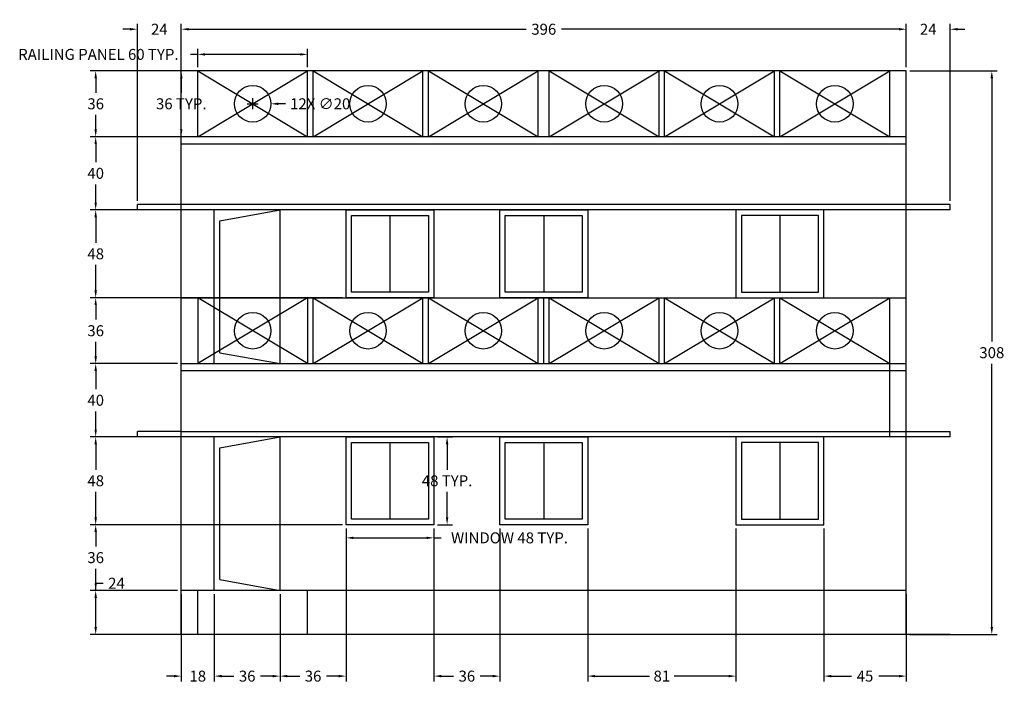
# Model space of a CAD drawing. Units: inches. Extents: x 853 to 2068, y 1026 to 2097.
# Tile 3 of 6: x 856 to 1394, y 1735 to 2097. Entities that reach past the tile are written whole.
import ezdxf

# ---------------------------------------------------------------- set-up
doc = ezdxf.new("R2010")
doc.units = ezdxf.units.IN
doc.header["$MEASUREMENT"] = 0
doc.layers.add('A-ANNO-DIMS', color=2, linetype='Continuous', lineweight=18)
doc.layers.add('A-ELEV', color=7, linetype='Continuous', lineweight=25)
doc.styles.get("Standard").update_dxf_attribs({"font": 'arial.ttf'})
doc.dimstyles.get("Standard").update_dxf_attribs({"dimtxt": 6, "dimasz": 4, "dimexe": 3, "dimexo": 2, "dimgap": 3, "dimtad": 0, "dimtih": 1, "dimtoh": 1, "dimdec": 0, "dimzin": 0, "dimdsep": 46, "dimlunit": 3, "dimtxsty": 'Standard', "dimcen": 3, "dimadec": 0, "dimazin": 0, "dimtfac": 1, "dimtdec": 0, "dimtofl": 0, "dimtmove": 0, "dimatfit": 3, "dimfxl": 1, "dimtolj": 1, "dimtzin": 0, "dimarcsym": 0})

# ---------------------------------------------------------------- blocks, each defined once
blk = doc.blocks.new('RAIL-PANEL')
for p, q in [((0, 36), (0, 0)), ((60, 36), (0, 0)), ((60, 0), (0, 36)), ((60, 36), (60, 0))]:
    blk.add_line(p, q)
blk.add_circle((30, 18), 10)
blk = doc.blocks.new('WIN-ELEV')
blk.add_line((24, 45), (24, 3))
for points in [[(0, 48), (48, 48), (48, 0), (0, 0)], [(3, 45), (45, 45), (45, 3), (3, 3)]]:
    blk.add_lwpolyline(points, close=True)
blk = doc.blocks.new('*D9')
at = {"layer": 'A-ANNO-DIMS', "color": 0, "lineweight": -2, "transparency": 16777216}
for p, q in [((1034.75, 1819.25), (1034.75, 1811.05)), ((1082.75, 1819.25), (1082.75, 1811.05)), ((1038.75, 1814.05), (1078.75, 1814.05)), ((1082.75, 1814.05), (1086.75, 1814.05))]:
    blk.add_line(p, q, dxfattribs=at)
at = {"layer": 'A-ANNO-DIMS', "color": 0, "transparency": 16777216}
for points in [[(1038.75, 1814.72), (1038.75, 1813.38), (1034.75, 1814.05)], [(1078.75, 1814.72), (1078.75, 1813.38), (1082.75, 1814.05)]]:
    blk.add_solid(points, dxfattribs=at)
at = {"layer": 'Defpoints', "color": 0, "transparency": 16777216}
for p in [(1034.75, 1821.25), (1082.75, 1821.25), (1082.75, 1814.05)]:
    blk.add_point(p, dxfattribs=at)
at = {"layer": 'A-ANNO-DIMS', "color": 0, "transparency": 16777216, "insert": (1124.03, 1814.05), "char_height": 6, "attachment_point": 5}
blk.add_mtext('\\A1;WINDOW 48 TYP.', dxfattribs=at)
blk = doc.blocks.new('*D10')
at = {"layer": 'A-ANNO-DIMS', "color": 0, "lineweight": -2, "transparency": 16777216}
for p, q in [((1084.75, 1869.25), (1092.95, 1869.25)), ((1089.95, 1865.25), (1089.95, 1851.31)), ((1089.95, 1825.25), (1089.95, 1839.19)), ((1084.75, 1821.25), (1092.95, 1821.25))]:
    blk.add_line(p, q, dxfattribs=at)
at = {"layer": 'A-ANNO-DIMS', "color": 0, "transparency": 16777216}
for points in [[(1089.28, 1865.25), (1090.62, 1865.25), (1089.95, 1869.25)], [(1089.28, 1825.25), (1090.62, 1825.25), (1089.95, 1821.25)]]:
    blk.add_solid(points, dxfattribs=at)
at = {"layer": 'Defpoints', "color": 0, "transparency": 16777216}
for p in [(1082.75, 1869.25), (1089.95, 1869.25), (1082.75, 1821.25)]:
    blk.add_point(p, dxfattribs=at)
at = {"layer": 'A-ANNO-DIMS', "color": 0, "transparency": 16777216, "insert": (1089.95, 1845.25), "char_height": 6, "attachment_point": 5}
blk.add_mtext('\\A1;48 TYP.', dxfattribs=at)
blk = doc.blocks.new('*D11')
at = {"layer": 'A-ANNO-DIMS', "color": 0, "lineweight": -2, "transparency": 16777216}
for p, q in [((953.75, 2078.25), (949.75, 2078.25)), ((953.75, 2071.25), (953.75, 2081.25)), ((1009.75, 2078.25), (957.75, 2078.25)), ((1013.75, 2071.25), (1013.75, 2081.25))]:
    blk.add_line(p, q, dxfattribs=at)
at = {"layer": 'A-ANNO-DIMS', "color": 0, "transparency": 16777216}
for points in [[(957.75, 2078.92), (957.75, 2077.58), (953.75, 2078.25)], [(1009.75, 2078.92), (1009.75, 2077.58), (1013.75, 2078.25)]]:
    blk.add_solid(points, dxfattribs=at)
at = {"layer": 'Defpoints', "color": 0, "transparency": 16777216}
for p in [(953.75, 2078.25), (953.75, 2069.25), (1013.75, 2069.25)]:
    blk.add_point(p, dxfattribs=at)
at = {"layer": 'A-ANNO-DIMS', "color": 0, "transparency": 16777216, "insert": (899.46, 2078.25), "char_height": 6, "attachment_point": 5}
blk.add_mtext('\\A1;RAILING PANEL 60 TYP.', dxfattribs=at)
blk = doc.blocks.new('*D12')
at = {"layer": 'A-ANNO-DIMS', "color": 0, "lineweight": -2, "transparency": 16777216}
for p, q in [((951.75, 2069.25), (941.75, 2069.25)), ((944.75, 2065.25), (944.75, 2057.32)), ((944.75, 2037.25), (944.75, 2045.19)), ((951.75, 2033.25), (941.75, 2033.25))]:
    blk.add_line(p, q, dxfattribs=at)
at = {"layer": 'A-ANNO-DIMS', "color": 0, "transparency": 16777216}
for points in [[(944.08, 2065.25), (945.42, 2065.25), (944.75, 2069.25)], [(944.08, 2037.25), (945.42, 2037.25), (944.75, 2033.25)]]:
    blk.add_solid(points, dxfattribs=at)
at = {"layer": 'Defpoints', "color": 0, "transparency": 16777216}
for p in [(953.75, 2069.25), (944.75, 2033.25), (953.75, 2033.25)]:
    blk.add_point(p, dxfattribs=at)
at = {"layer": 'A-ANNO-DIMS', "color": 0, "transparency": 16777216, "insert": (944.75, 2051.25), "char_height": 6, "attachment_point": 5}
blk.add_mtext('\\A1;36 TYP.', dxfattribs=at)
blk = doc.blocks.new('*D76')
at = {"layer": 'A-ANNO-DIMS', "color": 0, "lineweight": -2, "transparency": 16777216}
for p, q in [((898, 1785.25), (898, 1789.25)), ((898, 1789.25), (902, 1789.25)), ((942.75, 1785.25), (895, 1785.25)), ((898, 1765.25), (898, 1781.25)), ((942.75, 1761.25), (895, 1761.25))]:
    blk.add_line(p, q, dxfattribs=at)
at = {"layer": 'A-ANNO-DIMS', "color": 0, "transparency": 16777216}
for points in [[(897.33, 1781.25), (898.67, 1781.25), (898, 1785.25)], [(897.33, 1765.25), (898.67, 1765.25), (898, 1761.25)]]:
    blk.add_solid(points, dxfattribs=at)
at = {"layer": 'Defpoints', "color": 0, "transparency": 16777216}
for p in [(898, 1785.25), (944.75, 1785.25), (944.75, 1761.25)]:
    blk.add_point(p, dxfattribs=at)
at = {"layer": 'A-ANNO-DIMS', "color": 0, "transparency": 16777216, "insert": (909.34, 1789.25), "char_height": 6, "attachment_point": 5}
blk.add_mtext('\\A1;24', dxfattribs=at)
blk = doc.blocks.new('*D77')
at = {"layer": 'A-ANNO-DIMS', "color": 0, "lineweight": -2, "transparency": 16777216}
for p, q in [((1032.75, 1821.25), (895, 1821.25)), ((898, 1817.25), (898, 1809.32)), ((898, 1789.25), (898, 1797.19)), ((942.75, 1785.25), (895, 1785.25))]:
    blk.add_line(p, q, dxfattribs=at)
at = {"layer": 'A-ANNO-DIMS', "color": 0, "transparency": 16777216}
for points in [[(897.33, 1817.25), (898.67, 1817.25), (898, 1821.25)], [(897.33, 1789.25), (898.67, 1789.25), (898, 1785.25)]]:
    blk.add_solid(points, dxfattribs=at)
at = {"layer": 'Defpoints', "color": 0, "transparency": 16777216}
for p in [(898, 1821.25), (1034.75, 1821.25), (944.75, 1785.25)]:
    blk.add_point(p, dxfattribs=at)
at = {"layer": 'A-ANNO-DIMS', "color": 0, "transparency": 16777216, "insert": (898, 1803.25), "char_height": 6, "attachment_point": 5}
blk.add_mtext('\\A1;36', dxfattribs=at)
blk = doc.blocks.new('*D78')
at = {"layer": 'A-ANNO-DIMS', "color": 0, "lineweight": -2, "transparency": 16777216}
for p, q in [((942.75, 1869.25), (895, 1869.25)), ((898, 1865.25), (898, 1851.31)), ((898, 1825.25), (898, 1839.19)), ((1032.75, 1821.25), (895, 1821.25))]:
    blk.add_line(p, q, dxfattribs=at)
at = {"layer": 'A-ANNO-DIMS', "color": 0, "transparency": 16777216}
for points in [[(897.33, 1865.25), (898.67, 1865.25), (898, 1869.25)], [(897.33, 1825.25), (898.67, 1825.25), (898, 1821.25)]]:
    blk.add_solid(points, dxfattribs=at)
at = {"layer": 'Defpoints', "color": 0, "transparency": 16777216}
for p in [(898, 1869.25), (944.75, 1869.25), (1034.75, 1821.25)]:
    blk.add_point(p, dxfattribs=at)
at = {"layer": 'A-ANNO-DIMS', "color": 0, "transparency": 16777216, "insert": (898, 1845.25), "char_height": 6, "attachment_point": 5}
blk.add_mtext('\\A1;48', dxfattribs=at)
blk = doc.blocks.new('*D79')
at = {"layer": 'A-ANNO-DIMS', "color": 0, "lineweight": -2, "transparency": 16777216}
for p, q in [((942.75, 1909.25), (895, 1909.25)), ((898, 1905.25), (898, 1895.31)), ((898, 1873.25), (898, 1883.19)), ((942.75, 1869.25), (895, 1869.25))]:
    blk.add_line(p, q, dxfattribs=at)
at = {"layer": 'A-ANNO-DIMS', "color": 0, "transparency": 16777216}
for points in [[(897.33, 1905.25), (898.67, 1905.25), (898, 1909.25)], [(897.33, 1873.25), (898.67, 1873.25), (898, 1869.25)]]:
    blk.add_solid(points, dxfattribs=at)
at = {"layer": 'Defpoints', "color": 0, "transparency": 16777216}
for p in [(898, 1909.25), (944.75, 1909.25), (944.75, 1869.25)]:
    blk.add_point(p, dxfattribs=at)
at = {"layer": 'A-ANNO-DIMS', "color": 0, "transparency": 16777216, "insert": (898, 1889.25), "char_height": 6, "attachment_point": 5}
blk.add_mtext('\\A1;40', dxfattribs=at)
blk = doc.blocks.new('*D80')
at = {"layer": 'A-ANNO-DIMS', "color": 0, "lineweight": -2, "transparency": 16777216}
for p, q in [((1032.75, 1945.25), (895, 1945.25)), ((898, 1941.25), (898, 1933.32)), ((898, 1913.25), (898, 1921.19)), ((942.75, 1909.25), (895, 1909.25))]:
    blk.add_line(p, q, dxfattribs=at)
at = {"layer": 'A-ANNO-DIMS', "color": 0, "transparency": 16777216}
for points in [[(897.33, 1941.25), (898.67, 1941.25), (898, 1945.25)], [(897.33, 1913.25), (898.67, 1913.25), (898, 1909.25)]]:
    blk.add_solid(points, dxfattribs=at)
at = {"layer": 'Defpoints', "color": 0, "transparency": 16777216}
for p in [(898, 1945.25), (1034.75, 1945.25), (944.75, 1909.25)]:
    blk.add_point(p, dxfattribs=at)
at = {"layer": 'A-ANNO-DIMS', "color": 0, "transparency": 16777216, "insert": (898, 1927.25), "char_height": 6, "attachment_point": 5}
blk.add_mtext('\\A1;36', dxfattribs=at)
blk = doc.blocks.new('*D81')
at = {"layer": 'A-ANNO-DIMS', "color": 0, "lineweight": -2, "transparency": 16777216}
for p, q in [((942.75, 1993.25), (895, 1993.25)), ((898, 1989.25), (898, 1975.31)), ((898, 1949.25), (898, 1963.19)), ((1032.75, 1945.25), (895, 1945.25))]:
    blk.add_line(p, q, dxfattribs=at)
at = {"layer": 'A-ANNO-DIMS', "color": 0, "transparency": 16777216}
for points in [[(897.33, 1989.25), (898.67, 1989.25), (898, 1993.25)], [(897.33, 1949.25), (898.67, 1949.25), (898, 1945.25)]]:
    blk.add_solid(points, dxfattribs=at)
at = {"layer": 'Defpoints', "color": 0, "transparency": 16777216}
for p in [(898, 1993.25), (944.75, 1993.25), (1034.75, 1945.25)]:
    blk.add_point(p, dxfattribs=at)
at = {"layer": 'A-ANNO-DIMS', "color": 0, "transparency": 16777216, "insert": (898, 1969.25), "char_height": 6, "attachment_point": 5}
blk.add_mtext('\\A1;48', dxfattribs=at)
blk = doc.blocks.new('*D82')
at = {"layer": 'A-ANNO-DIMS', "color": 0, "lineweight": -2, "transparency": 16777216}
for p, q in [((942.75, 2033.25), (895, 2033.25)), ((898, 2029.25), (898, 2019.31)), ((898, 1997.25), (898, 2007.19)), ((942.75, 1993.25), (895, 1993.25))]:
    blk.add_line(p, q, dxfattribs=at)
at = {"layer": 'A-ANNO-DIMS', "color": 0, "transparency": 16777216}
for points in [[(897.33, 2029.25), (898.67, 2029.25), (898, 2033.25)], [(897.33, 1997.25), (898.67, 1997.25), (898, 1993.25)]]:
    blk.add_solid(points, dxfattribs=at)
at = {"layer": 'Defpoints', "color": 0, "transparency": 16777216}
for p in [(898, 2033.25), (944.75, 2033.25), (944.75, 1993.25)]:
    blk.add_point(p, dxfattribs=at)
at = {"layer": 'A-ANNO-DIMS', "color": 0, "transparency": 16777216, "insert": (898, 2013.25), "char_height": 6, "attachment_point": 5}
blk.add_mtext('\\A1;40', dxfattribs=at)
blk = doc.blocks.new('*D83')
at = {"layer": 'A-ANNO-DIMS', "color": 0, "lineweight": -2, "transparency": 16777216}
for p, q in [((942.75, 2069.25), (895, 2069.25)), ((898, 2065.25), (898, 2057.32)), ((898, 2037.25), (898, 2045.19)), ((942.75, 2033.25), (895, 2033.25))]:
    blk.add_line(p, q, dxfattribs=at)
at = {"layer": 'A-ANNO-DIMS', "color": 0, "transparency": 16777216}
for points in [[(897.33, 2065.25), (898.67, 2065.25), (898, 2069.25)], [(897.33, 2037.25), (898.67, 2037.25), (898, 2033.25)]]:
    blk.add_solid(points, dxfattribs=at)
at = {"layer": 'Defpoints', "color": 0, "transparency": 16777216}
for p in [(898, 2069.25), (944.75, 2069.25), (944.75, 2033.25)]:
    blk.add_point(p, dxfattribs=at)
at = {"layer": 'A-ANNO-DIMS', "color": 0, "transparency": 16777216, "insert": (898, 2051.25), "char_height": 6, "attachment_point": 5}
blk.add_mtext('\\A1;36', dxfattribs=at)
blk = doc.blocks.new('*D84')
at = {"layer": 'A-ANNO-DIMS', "color": 0, "lineweight": -2, "transparency": 16777216}
for p, q in [((1342.75, 2069.25), (1390.5, 2069.25)), ((1387.5, 2065.25), (1387.5, 1921.32)), ((1387.5, 1765.25), (1387.5, 1909.19)), ((1342.75, 1761.25), (1390.5, 1761.25))]:
    blk.add_line(p, q, dxfattribs=at)
at = {"layer": 'A-ANNO-DIMS', "color": 0, "transparency": 16777216}
for points in [[(1386.83, 2065.25), (1388.17, 2065.25), (1387.5, 2069.25)], [(1386.83, 1765.25), (1388.17, 1765.25), (1387.5, 1761.25)]]:
    blk.add_solid(points, dxfattribs=at)
at = {"layer": 'Defpoints', "color": 0, "transparency": 16777216}
for p in [(1340.75, 2069.25), (1387.5, 2069.25), (1340.75, 1761.25)]:
    blk.add_point(p, dxfattribs=at)
at = {"layer": 'A-ANNO-DIMS', "color": 0, "transparency": 16777216, "insert": (1387.5, 1915.25), "char_height": 6, "attachment_point": 5}
blk.add_mtext('\\A1;308', dxfattribs=at)
blk = doc.blocks.new('*D85')
at = {"layer": 'A-ANNO-DIMS', "color": 0, "lineweight": -2, "transparency": 16777216}
for p, q in [((944.75, 1783.25), (944.75, 1735.5)), ((962.75, 1783.25), (962.75, 1735.5)), ((940.75, 1738.5), (936.75, 1738.5)), ((966.75, 1738.5), (970.75, 1738.5))]:
    blk.add_line(p, q, dxfattribs=at)
at = {"layer": 'A-ANNO-DIMS', "color": 0, "transparency": 16777216}
for points in [[(940.75, 1739.17), (940.75, 1737.83), (944.75, 1738.5)], [(966.75, 1739.17), (966.75, 1737.83), (962.75, 1738.5)]]:
    blk.add_solid(points, dxfattribs=at)
at = {"layer": 'Defpoints', "color": 0, "transparency": 16777216}
for p in [(944.75, 1785.25), (962.75, 1785.25), (962.75, 1738.5)]:
    blk.add_point(p, dxfattribs=at)
at = {"layer": 'A-ANNO-DIMS', "color": 0, "transparency": 16777216, "insert": (953.75, 1738.5), "char_height": 6, "attachment_point": 5}
blk.add_mtext('\\A1;18', dxfattribs=at)
blk = doc.blocks.new('*D86')
at = {"layer": 'A-ANNO-DIMS', "color": 0, "lineweight": -2, "transparency": 16777216}
for p, q in [((962.75, 1783.25), (962.75, 1735.5)), ((998.75, 1783.25), (998.75, 1735.5)), ((966.75, 1738.5), (973.46, 1738.5)), ((994.75, 1738.5), (988.04, 1738.5))]:
    blk.add_line(p, q, dxfattribs=at)
at = {"layer": 'A-ANNO-DIMS', "color": 0, "transparency": 16777216}
for points in [[(966.75, 1739.17), (966.75, 1737.83), (962.75, 1738.5)], [(994.75, 1739.17), (994.75, 1737.83), (998.75, 1738.5)]]:
    blk.add_solid(points, dxfattribs=at)
at = {"layer": 'Defpoints', "color": 0, "transparency": 16777216}
for p in [(962.75, 1785.25), (998.75, 1785.25), (998.75, 1738.5)]:
    blk.add_point(p, dxfattribs=at)
at = {"layer": 'A-ANNO-DIMS', "color": 0, "transparency": 16777216, "insert": (980.75, 1738.5), "char_height": 6, "attachment_point": 5}
blk.add_mtext('\\A1;36', dxfattribs=at)
blk = doc.blocks.new('*D87')
at = {"layer": 'A-ANNO-DIMS', "color": 0, "lineweight": -2, "transparency": 16777216}
for p, q in [((1034.75, 1819.25), (1034.75, 1735.5)), ((998.75, 1783.25), (998.75, 1735.5)), ((1002.75, 1738.5), (1009.46, 1738.5)), ((1030.75, 1738.5), (1024.04, 1738.5))]:
    blk.add_line(p, q, dxfattribs=at)
at = {"layer": 'A-ANNO-DIMS', "color": 0, "transparency": 16777216}
for points in [[(1002.75, 1739.17), (1002.75, 1737.83), (998.75, 1738.5)], [(1030.75, 1739.17), (1030.75, 1737.83), (1034.75, 1738.5)]]:
    blk.add_solid(points, dxfattribs=at)
at = {"layer": 'Defpoints', "color": 0, "transparency": 16777216}
for p in [(1034.75, 1821.25), (998.75, 1785.25), (1034.75, 1738.5)]:
    blk.add_point(p, dxfattribs=at)
at = {"layer": 'A-ANNO-DIMS', "color": 0, "transparency": 16777216, "insert": (1016.75, 1738.5), "char_height": 6, "attachment_point": 5}
blk.add_mtext('\\A1;36', dxfattribs=at)
blk = doc.blocks.new('*D88')
at = {"layer": 'A-ANNO-DIMS', "color": 0, "lineweight": -2, "transparency": 16777216}
for p, q in [((1082.75, 1819.25), (1082.75, 1735.5)), ((1118.75, 1819.25), (1118.75, 1735.5)), ((1086.75, 1738.5), (1093.46, 1738.5)), ((1114.75, 1738.5), (1108.04, 1738.5))]:
    blk.add_line(p, q, dxfattribs=at)
at = {"layer": 'A-ANNO-DIMS', "color": 0, "transparency": 16777216}
for points in [[(1086.75, 1739.17), (1086.75, 1737.83), (1082.75, 1738.5)], [(1114.75, 1739.17), (1114.75, 1737.83), (1118.75, 1738.5)]]:
    blk.add_solid(points, dxfattribs=at)
at = {"layer": 'Defpoints', "color": 0, "transparency": 16777216}
for p in [(1082.75, 1821.25), (1118.75, 1821.25), (1118.75, 1738.5)]:
    blk.add_point(p, dxfattribs=at)
at = {"layer": 'A-ANNO-DIMS', "color": 0, "transparency": 16777216, "insert": (1100.75, 1738.5), "char_height": 6, "attachment_point": 5}
blk.add_mtext('\\A1;36', dxfattribs=at)
blk = doc.blocks.new('*D89')
at = {"layer": 'A-ANNO-DIMS', "color": 0, "lineweight": -2, "transparency": 16777216}
for p, q in [((1166.75, 1819.25), (1166.75, 1735.5)), ((1247.75, 1819.25), (1247.75, 1735.5)), ((1170.75, 1738.5), (1200.53, 1738.5)), ((1243.75, 1738.5), (1213.97, 1738.5))]:
    blk.add_line(p, q, dxfattribs=at)
at = {"layer": 'A-ANNO-DIMS', "color": 0, "transparency": 16777216}
for points in [[(1170.75, 1739.17), (1170.75, 1737.83), (1166.75, 1738.5)], [(1243.75, 1739.17), (1243.75, 1737.83), (1247.75, 1738.5)]]:
    blk.add_solid(points, dxfattribs=at)
at = {"layer": 'Defpoints', "color": 0, "transparency": 16777216}
for p in [(1166.75, 1821.25), (1247.75, 1821.25), (1247.75, 1738.5)]:
    blk.add_point(p, dxfattribs=at)
at = {"layer": 'A-ANNO-DIMS', "color": 0, "transparency": 16777216, "insert": (1207.25, 1738.5), "char_height": 6, "attachment_point": 5}
blk.add_mtext('\\A1;81', dxfattribs=at)
blk = doc.blocks.new('*D90')
at = {"layer": 'A-ANNO-DIMS', "color": 0, "lineweight": -2, "transparency": 16777216}
for p, q in [((1295.75, 1819.25), (1295.75, 1735.5)), ((1340.75, 1783.25), (1340.75, 1735.5)), ((1299.75, 1738.5), (1310.81, 1738.5)), ((1336.75, 1738.5), (1325.69, 1738.5))]:
    blk.add_line(p, q, dxfattribs=at)
at = {"layer": 'A-ANNO-DIMS', "color": 0, "transparency": 16777216}
for points in [[(1299.75, 1739.17), (1299.75, 1737.83), (1295.75, 1738.5)], [(1336.75, 1739.17), (1336.75, 1737.83), (1340.75, 1738.5)]]:
    blk.add_solid(points, dxfattribs=at)
at = {"layer": 'Defpoints', "color": 0, "transparency": 16777216}
for p in [(1295.75, 1821.25), (1340.75, 1785.25), (1340.75, 1738.5)]:
    blk.add_point(p, dxfattribs=at)
at = {"layer": 'A-ANNO-DIMS', "color": 0, "transparency": 16777216, "insert": (1318.25, 1738.5), "char_height": 6, "attachment_point": 5}
blk.add_mtext('\\A1;45', dxfattribs=at)
blk = doc.blocks.new('*D91')
at = {"layer": 'A-ANNO-DIMS', "color": 0, "lineweight": -2, "transparency": 16777216}
for p, q in [((920.75, 1998.25), (920.75, 2095)), ((944.75, 1995.25), (944.75, 2095)), ((916.75, 2092), (912.75, 2092)), ((948.75, 2092), (952.75, 2092))]:
    blk.add_line(p, q, dxfattribs=at)
at = {"layer": 'A-ANNO-DIMS', "color": 0, "transparency": 16777216}
for points in [[(916.75, 2092.67), (916.75, 2091.33), (920.75, 2092)], [(948.75, 2092.67), (948.75, 2091.33), (944.75, 2092)]]:
    blk.add_solid(points, dxfattribs=at)
at = {"layer": 'Defpoints', "color": 0, "transparency": 16777216}
for p in [(944.75, 2092), (920.75, 1996.25), (944.75, 1993.25)]:
    blk.add_point(p, dxfattribs=at)
at = {"layer": 'A-ANNO-DIMS', "color": 0, "transparency": 16777216, "insert": (932.75, 2092), "char_height": 6, "attachment_point": 5}
blk.add_mtext('\\A1;24', dxfattribs=at)
blk = doc.blocks.new('*D92')
at = {"layer": 'A-ANNO-DIMS', "color": 0, "lineweight": -2, "transparency": 16777216}
for p, q in [((944.75, 2071.25), (944.75, 2095)), ((1340.75, 2071.25), (1340.75, 2095)), ((948.75, 2092), (1133.13, 2092)), ((1336.75, 2092), (1152.38, 2092))]:
    blk.add_line(p, q, dxfattribs=at)
at = {"layer": 'A-ANNO-DIMS', "color": 0, "transparency": 16777216}
for points in [[(948.75, 2092.67), (948.75, 2091.33), (944.75, 2092)], [(1336.75, 2092.67), (1336.75, 2091.33), (1340.75, 2092)]]:
    blk.add_solid(points, dxfattribs=at)
at = {"layer": 'Defpoints', "color": 0, "transparency": 16777216}
for p in [(1340.75, 2092), (944.75, 2069.25), (1340.75, 2069.25)]:
    blk.add_point(p, dxfattribs=at)
at = {"layer": 'A-ANNO-DIMS', "color": 0, "transparency": 16777216, "insert": (1142.75, 2092), "char_height": 6, "attachment_point": 5}
blk.add_mtext('\\A1;396', dxfattribs=at)
blk = doc.blocks.new('*D93')
at = {"layer": 'A-ANNO-DIMS', "color": 0, "lineweight": -2, "transparency": 16777216}
for p, q in [((1340.75, 2071.25), (1340.75, 2095)), ((1364.75, 1998.25), (1364.75, 2095)), ((1336.75, 2092), (1332.75, 2092)), ((1368.75, 2092), (1372.75, 2092))]:
    blk.add_line(p, q, dxfattribs=at)
at = {"layer": 'A-ANNO-DIMS', "color": 0, "transparency": 16777216}
for points in [[(1336.75, 2092.67), (1336.75, 2091.33), (1340.75, 2092)], [(1368.75, 2092.67), (1368.75, 2091.33), (1364.75, 2092)]]:
    blk.add_solid(points, dxfattribs=at)
at = {"layer": 'Defpoints', "color": 0, "transparency": 16777216}
for p in [(1364.75, 2092), (1340.75, 2069.25), (1364.75, 1996.25)]:
    blk.add_point(p, dxfattribs=at)
at = {"layer": 'A-ANNO-DIMS', "color": 0, "transparency": 16777216, "insert": (1352.75, 2092), "char_height": 6, "attachment_point": 5}
blk.add_mtext('\\A1;24', dxfattribs=at)
blk = doc.blocks.new('*D121')
at = {"layer": 'A-ANNO-DIMS', "color": 0, "lineweight": -2, "transparency": 16777216}
for p, q in [((980.75, 2051.25), (986.75, 2051.25)), ((983.75, 2048.25), (983.75, 2054.25)), ((1001.75, 2051.25), (997.75, 2051.25))]:
    blk.add_line(p, q, dxfattribs=at)
at = {"layer": 'A-ANNO-DIMS', "color": 0, "transparency": 16777216}
blk.add_solid([(997.75, 2051.92), (997.75, 2050.58), (993.75, 2051.25)], dxfattribs=at)
at = {"layer": 'Defpoints', "color": 0, "transparency": 16777216}
for p in [(973.75, 2051.25), (993.75, 2051.25)]:
    blk.add_point(p, dxfattribs=at)
at = {"layer": 'A-ANNO-DIMS', "color": 0, "transparency": 16777216, "insert": (1020.64, 2051.25), "char_height": 6, "attachment_point": 5}
blk.add_mtext('\\A1;12X ∅20', dxfattribs=at)

msp = doc.modelspace()

# ---------------------------------------------------------------- linework, layer by layer
at = {"layer": 'A-ELEV'}
for p, q in [((944.751, 1761.2513), (944.751, 2069.2513)), ((1340.751, 2069.2513), (944.751, 2069.2513)), ((1340.751, 1761.2513), (1340.751, 2069.2513)), ((1340.751, 2033.2513), (944.751, 2033.2513)), ((1340.751, 2029.2513), (944.751, 2029.2513)), ((1364.751, 1996.2513), (920.751, 1996.2513)), ((920.751, 1993.2513), (920.751, 1996.2513)), ((1364.751, 1993.2513), (1364.751, 1996.2513)), ((944.751, 1993.2513), (920.751, 1993.2513)), ((1364.751, 1993.2513), (944.751, 1993.2513)), ((962.751, 1909.2513), (962.751, 1993.2513)), ((965.751, 1987.2513), (998.751, 1993.2513)), ((998.751, 1909.2513), (998.751, 1993.2513)), ((965.751, 1915.2513), (965.751, 1987.2513)), ((944.751, 1945.2513), (1340.751, 1945.2513)), ((1142.751, 1909.2513), (1142.751, 1945.2513)), ((1271.751, 1909.2513), (1271.751, 1945.2513)), ((1271.751, 1909.2513), (1331.751, 1945.2513)), ((1271.751, 1945.2513), (1331.751, 1909.2513)), ((1331.751, 1869.2513), (1331.751, 1945.2513)), ((965.751, 1915.2513), (998.751, 1909.2513)), ((944.751, 1909.2513), (1340.751, 1909.2513)), ((1340.751, 1905.2513), (944.751, 1905.2513)), ((920.751, 1869.2513), (920.751, 1872.2513)), ((944.751, 1872.2513), (920.751, 1872.2513)), ((944.751, 1872.2513), (1364.751, 1872.2513)), ((1364.751, 1869.2513), (1364.751, 1872.2513)), ((944.751, 1869.2513), (920.751, 1869.2513)), ((1364.751, 1869.2513), (944.751, 1869.2513)), ((962.751, 1785.2513), (962.751, 1869.2513)), ((965.751, 1863.2513), (998.751, 1869.2513)), ((998.751, 1785.2513), (998.751, 1869.2513)), ((965.751, 1791.2513), (965.751, 1863.2513)), ((965.751, 1791.2513), (998.751, 1785.2513)), ((1340.751, 1785.2513), (944.751, 1785.2513)), ((953.751, 1761.2513), (953.751, 1785.2513)), ((1013.751, 1761.2513), (1013.751, 1785.2513)), ((1364.751, 1761.2513), (920.751, 1761.2513))]:
    msp.add_line(p, q, dxfattribs=at)
msp.add_circle((1301.751, 1927.2513), 10, dxfattribs=at)

# ---------------------------------------------------------------- block references
at = {"layer": 'A-ELEV', "rotation": 180}
for p in [(1013.751, 2069.2515), (1076.751, 2069.2515), (1139.751, 2069.2515), (1205.751, 2069.2515), (1268.751, 2069.2515), (1331.751, 2069.2515), (1076.751, 1945.2515), (1139.751, 1945.2515), (1205.751, 1945.2515), (1268.751, 1945.2515)]:
    msp.add_blockref('RAIL-PANEL', p, dxfattribs=at)
at = {"layer": 'A-ELEV'}
for name, p in [('WIN-ELEV', (1034.751, 1945.251)), ('WIN-ELEV', (1118.751, 1945.251)), ('RAIL-PANEL', (953.751, 1909.251)), ('WIN-ELEV', (1034.751, 1821.251)), ('WIN-ELEV', (1118.751, 1821.251))]:
    msp.add_blockref(name, p, dxfattribs=at)
at = {"layer": 'A-ELEV', "extrusion": (0, 0, -1), "zscale": -1}
for p in [(-1295.751, 1945.251), (-1295.751, 1821.251)]:
    msp.add_blockref('WIN-ELEV', p, dxfattribs=at)

# ---------------------------------------------------------------- dimensions: what is measured, and where the dimension line sits
at = {"layer": 'A-ANNO-DIMS'}
for base, p1, p2, angle, text, picture, middle in [((953.751, 2078.2513), (1013.751, 2069.2513), (953.751, 2069.2513), 180, 'RAILING PANEL <> TYP.', '*D11', (899.4632, 2078.2513)), ((944.751, 2033.2513), (953.751, 2069.2513), (953.751, 2033.2513), 270, '<> TYP.', '*D12', (944.751, 2051.2513)), ((1089.951, 1869.2513), (1082.751, 1821.2513), (1082.751, 1869.2513), 90, '<> TYP.', '*D10', (1089.951, 1845.2513))]:
    dim = msp.add_linear_dim(base=base, p1=p1, p2=p2, angle=angle, text=text, dimstyle='Standard', override={"dimdec": 0, "dimrnd": 0, "dimzin": 0, "dimlunit": 2}, dxfattribs=at)
    dim.commit()
    dim.dimension.update_dxf_attribs({"geometry": picture, "text_midpoint": middle})
for base, p1, p2, picture, middle in [((944.751, 2092.0013), (920.751, 1996.2513), (944.751, 1993.2513), '*D91', (932.751, 2092.0013)), ((1340.751, 2092.0013), (944.751, 2069.2513), (1340.751, 2069.2513), '*D92', (1142.751, 2092.0013)), ((1364.751, 2092.0013), (1340.751, 2069.2513), (1364.751, 1996.2513), '*D93', (1352.751, 2092.0013)), ((1034.751, 1738.5013), (998.751, 1785.2513), (1034.751, 1821.2513), '*D87', (1016.751, 1738.5013)), ((1118.751, 1738.5013), (1082.751, 1821.2513), (1118.751, 1821.2513), '*D88', (1100.751, 1738.5013)), ((1247.751, 1738.5013), (1166.751, 1821.2513), (1247.751, 1821.2513), '*D89', (1207.251, 1738.5013)), ((1340.751, 1738.5013), (1295.751, 1821.2513), (1340.751, 1785.2513), '*D90', (1318.251, 1738.5013)), ((962.751, 1738.5013), (944.751, 1785.2513), (962.751, 1785.2513), '*D85', (953.751, 1738.5013)), ((998.751, 1738.5013), (962.751, 1785.2513), (998.751, 1785.2513), '*D86', (980.751, 1738.5013))]:
    dim = msp.add_linear_dim(base=base, p1=p1, p2=p2, dimstyle='Standard', override={"dimdec": 0, "dimlfac": 1, "dimrnd": 0, "dimzin": 0, "dimdsep": 46, "dimlunit": 2}, dxfattribs=at)
    dim.commit()
    dim.dimension.update_dxf_attribs({"geometry": picture, "text_midpoint": middle})
for base, p1, p2, picture, middle in [((898.001, 2069.2513), (944.751, 2033.2513), (944.751, 2069.2513), '*D83', (898.001, 2051.2513)), ((1387.501, 2069.2513), (1340.751, 1761.2513), (1340.751, 2069.2513), '*D84', (1387.501, 1915.2513)), ((898.001, 2033.2513), (944.751, 1993.2513), (944.751, 2033.2513), '*D82', (898.001, 2013.2513)), ((898.001, 1993.2513), (1034.751, 1945.2513), (944.751, 1993.2513), '*D81', (898.001, 1969.2513)), ((898.001, 1945.2513), (944.751, 1909.2513), (1034.751, 1945.2513), '*D80', (898.001, 1927.2513)), ((898.001, 1909.2513), (944.751, 1869.2513), (944.751, 1909.2513), '*D79', (898.001, 1889.2513)), ((898.001, 1869.2513), (1034.751, 1821.2513), (944.751, 1869.2513), '*D78', (898.001, 1845.2513)), ((898.001, 1821.2513), (944.751, 1785.2513), (1034.751, 1821.2513), '*D77', (898.001, 1803.2513)), ((898.001, 1785.2513), (944.751, 1761.2513), (944.751, 1785.2513), '*D76', (909.3373, 1789.2513))]:
    dim = msp.add_linear_dim(base=base, p1=p1, p2=p2, angle=90, dimstyle='Standard', override={"dimdec": 0, "dimlfac": 1, "dimrnd": 0, "dimzin": 0, "dimdsep": 46, "dimlunit": 2}, dxfattribs=at)
    dim.commit()
    dim.dimension.update_dxf_attribs({"geometry": picture, "text_midpoint": middle})
dim = msp.add_diameter_dim_2p(p1=(973.751, 2051.2515), p2=(993.751, 2051.251), text='12X <>', dimstyle='Standard', override={"dimdec": 0, "dimlfac": 1, "dimrnd": 0, "dimzin": 0, "dimdsep": 46, "dimlunit": 2}, dxfattribs=at)
dim.commit()
dim.dimension.update_dxf_attribs({"geometry": '*D121', "text_midpoint": (1001.751, 2051.2508), "dimtype": 163})
dim = msp.add_linear_dim(base=(1082.751, 1814.0513), p1=(1034.751, 1821.2513), p2=(1082.751, 1821.2513), text='WINDOW <> TYP.', dimstyle='Standard', override={"dimdec": 0, "dimrnd": 0, "dimzin": 0, "dimlunit": 2}, dxfattribs=at)
dim.commit()
dim.dimension.update_dxf_attribs({"geometry": '*D9', "text_midpoint": (1124.03, 1814.0513)})

doc.saveas('drawing.dxf')
